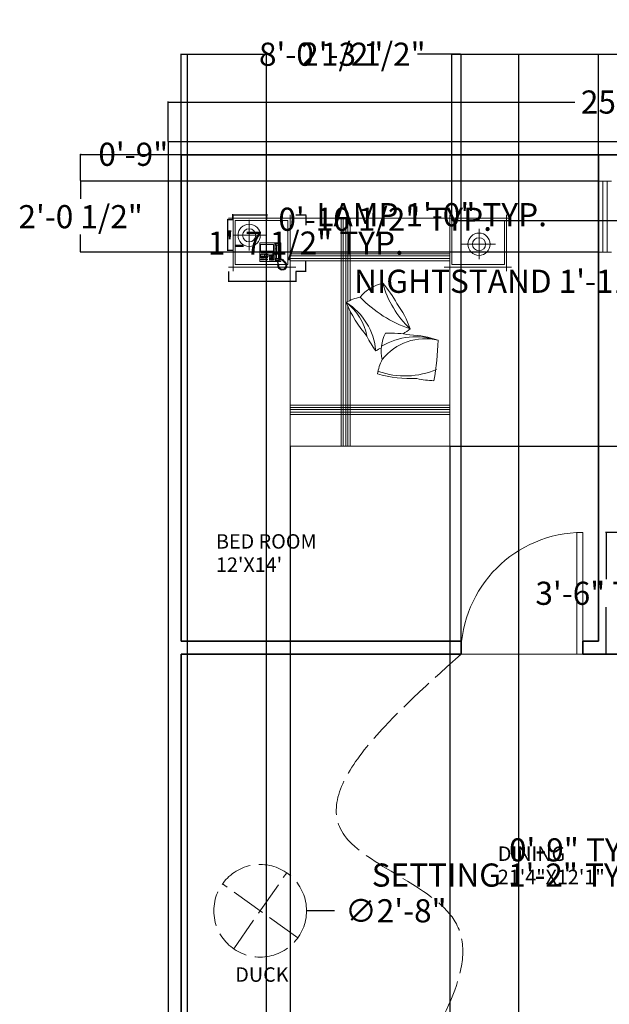
# Model space of a CAD drawing. Units: inches. Extents: x -26 to 385, y 12 to 697.
# Tile 12 of 13: x -26 to 177, y 356 to 697. Entities that reach past the tile are written whole.
import ezdxf

# ---------------------------------------------------------------- set-up
doc = ezdxf.new("R2010")
doc.units = ezdxf.units.IN
doc.header["$MEASUREMENT"] = 0
doc.linetypes.add('ACAD_ISO02W100', pattern=[15, 12, -3])
for name, color, linetype, lineweight in [('A-ANNO-DIMS', 4, 'Continuous', 18), ('A-AREA-IDEN', 4, 'Continuous', 18), ('A-DOOR', 30, 'Continuous', 20), ('A-EQPM', 210, 'Continuous', 13), ('A-FLOR-OVHD', 3, 'ACAD_ISO02W100', 13), ('A-GLAZ', 5, 'Continuous', 18), ('A-WALL', 40, 'Continuous', 35), ('C-PROP', 40, 'Continuous', 25), ('Furniture', 210, 'Continuous', 15)]:
    doc.layers.add(name, color=color, linetype=linetype, lineweight=lineweight)
doc.styles.get("Standard").update_dxf_attribs({"font": 'italic8.shx'})
doc.dimstyles.get("Standard").update_dxf_attribs({"dimtxt": 8, "dimasz": 0.18, "dimexe": 0.18, "dimexo": 0.0625, "dimgap": 0.09, "dimtad": 0, "dimtih": 1, "dimtoh": 1, "dimdec": 4, "dimzin": 0, "dimdsep": 46, "dimlunit": 3, "dimtxsty": 'Standard', "dimcen": 0.09, "dimclrd": 2, "dimclre": 3, "dimclrt": 6, "dimadec": 0, "dimazin": 0, "dimtfac": 1, "dimtdec": 4, "dimtofl": 0, "dimtmove": 0, "dimatfit": 3, "dimfxl": 1, "dimtolj": 1, "dimtzin": 0, "dimarcsym": 0})

# ---------------------------------------------------------------- blocks, each defined once
blk = doc.blocks.new('*D1')
at = {"layer": 'A-ANNO-DIMS', "color": 0, "lineweight": -2, "transparency": 16777216}
for p, q in [((25.13, 654.44), (25.13, 668.29)), ((25.31, 668.11), (165.52, 668.11)), ((324.95, 668.11), (184.74, 668.11)), ((325.13, 654.44), (325.13, 668.29))]:
    blk.add_line(p, q, dxfattribs=at)
at = {"layer": 'A-ANNO-DIMS', "color": 0, "transparency": 16777216}
for points in [[(25.31, 668.14), (25.31, 668.08), (25.13, 668.11)], [(324.95, 668.14), (324.95, 668.08), (325.13, 668.11)]]:
    blk.add_solid(points, dxfattribs=at)
at = {"layer": 'Defpoints', "color": 0, "transparency": 16777216}
for p in [(325.13, 668.11), (25.13, 654.38), (325.13, 654.38)]:
    blk.add_point(p, dxfattribs=at)
at = {"layer": 'A-ANNO-DIMS', "color": 0, "transparency": 16777216, "insert": (175.13, 668.11), "char_height": 8, "attachment_point": 5}
blk.add_mtext("\\A1;25'", dxfattribs=at)
blk = doc.blocks.new('DOOR-SWING-42IN')
for p, q in [((0, 0), (0, 42)), ((2, 0), (2, 42)), ((42, 0), (0, 0))]:
    blk.add_line(p, q)
blk.add_arc((0, 0), 42, 0, 90)
blk = doc.blocks.new('LAMP-BEDSIDE')
for p, q in [((0, -5.2), (0, 5.37)), ((-5.64, 0), (6.16, 0))]:
    blk.add_line(p, q)
for radius in [3.85, 2.27]:
    blk.add_circle((0, 0), radius)
blk = doc.blocks.new('NIGHTSTAND')
for p, q in [((-0.72, 17.12), (-0.72, -2.31)), ((18.22, 15.18), (0, 15.18)), ((0, 15.18), (0, 0)), ((18.22, 0), (18.22, 15.18)), ((0, 0), (18.22, 0)), ((-2.34, -0.93), (20.89, -0.93))]:
    blk.add_line(p, q)
blk = doc.blocks.new('*D15')
at = {"layer": 'A-ANNO-DIMS', "color": 3, "lineweight": -2, "transparency": 16777216}
for p, q in [((221.9, 409.73), (222.99, 407.84)), ((209.98, 402.84), (211.07, 400.96))]:
    blk.add_line(p, q, dxfattribs=at)
at = {"layer": 'A-ANNO-DIMS', "color": 2, "lineweight": -2, "transparency": 16777216}
for p, q in [((222.74, 407.9), (211.14, 401.2)), ((210.82, 401.02), (210.64, 401.02)), ((210.98, 401.11), (210.82, 401.02))]:
    blk.add_line(p, q, dxfattribs=at)
at = {"layer": 'A-ANNO-DIMS', "color": 2, "transparency": 16777216}
for points in [[(222.73, 407.93), (222.76, 407.88), (222.9, 407.99)], [(211.12, 401.23), (211.15, 401.18), (210.98, 401.11)]]:
    blk.add_solid(points, dxfattribs=at)
at = {"layer": 'Defpoints', "color": 0, "transparency": 16777216}
for p in [(221.87, 409.78), (209.95, 402.9), (210.98, 401.11)]:
    blk.add_point(p, dxfattribs=at)
at = {"layer": 'A-ANNO-DIMS', "color": 6, "transparency": 16777216, "insert": (143.32, 401.02), "char_height": 8, "attachment_point": 5}
blk.add_mtext('\\A1;SETTING 1\'-2" TYP.', dxfattribs=at)
blk = doc.blocks.new('*D16')
at = {"layer": 'A-ANNO-DIMS', "color": 2, "lineweight": -2, "transparency": 16777216}
for p, q in [((203.62, 409.73), (203.44, 409.73)), ((203.71, 409.58), (203.62, 409.73)), ((208.07, 402.02), (203.8, 409.42))]:
    blk.add_line(p, q, dxfattribs=at)
at = {"layer": 'A-ANNO-DIMS', "color": 3, "lineweight": -2, "transparency": 16777216}
for p, q in [((205.44, 410.58), (203.55, 409.49)), ((209.89, 402.87), (208, 401.78))]:
    blk.add_line(p, q, dxfattribs=at)
at = {"layer": 'A-ANNO-DIMS', "color": 2, "transparency": 16777216}
for points in [[(203.82, 409.44), (203.77, 409.41), (203.71, 409.58)], [(208.1, 402.04), (208.04, 402.01), (208.16, 401.87)]]:
    blk.add_solid(points, dxfattribs=at)
at = {"layer": 'Defpoints', "color": 0, "transparency": 16777216}
for p in [(203.71, 409.58), (205.5, 410.61), (209.95, 402.9)]:
    blk.add_point(p, dxfattribs=at)
at = {"layer": 'A-ANNO-DIMS', "color": 6, "transparency": 16777216, "insert": (167.16, 409.73), "char_height": 8, "attachment_point": 5}
blk.add_mtext('\\A1;0\'-9" TYP.', dxfattribs=at)
blk = doc.blocks.new('*D20')
at = {"layer": 'A-ANNO-DIMS', "color": 3, "lineweight": -2, "transparency": 16777216}
for p, q in [((182.53, 519.38), (176.11, 519.38)), ((182.53, 477.38), (176.11, 477.38))]:
    blk.add_line(p, q, dxfattribs=at)
at = {"layer": 'A-ANNO-DIMS', "color": 2, "lineweight": -2, "transparency": 16777216}
for p, q in [((176.29, 519.2), (176.29, 503.23)), ((176.29, 477.56), (176.29, 493.53))]:
    blk.add_line(p, q, dxfattribs=at)
at = {"layer": 'A-ANNO-DIMS', "color": 2, "transparency": 16777216}
for points in [[(176.26, 519.2), (176.32, 519.2), (176.29, 519.38)], [(176.26, 477.56), (176.32, 477.56), (176.29, 477.38)]]:
    blk.add_solid(points, dxfattribs=at)
at = {"layer": 'Defpoints', "color": 0, "transparency": 16777216}
for p in [(176.29, 519.38), (182.59, 519.38), (182.59, 477.38)]:
    blk.add_point(p, dxfattribs=at)
at = {"layer": 'A-ANNO-DIMS', "color": 6, "transparency": 16777216, "insert": (176.29, 498.38), "char_height": 8, "attachment_point": 5}
blk.add_mtext('\\A1;3\'-6" TYP.', dxfattribs=at)
blk = doc.blocks.new('*D21')
at = {"layer": 'A-ANNO-DIMS', "color": 3, "lineweight": -2, "transparency": 16777216}
for p, q in [((45.89, 609.6), (45.89, 606)), ((69.11, 609.6), (69.11, 606))]:
    blk.add_line(p, q, dxfattribs=at)
at = {"layer": 'A-ANNO-DIMS', "color": 2, "lineweight": -2, "transparency": 16777216}
for p, q in [((46.07, 606.18), (68.93, 606.18)), ((69.11, 606.18), (69.29, 606.18))]:
    blk.add_line(p, q, dxfattribs=at)
at = {"layer": 'A-ANNO-DIMS', "color": 2, "transparency": 16777216}
for points in [[(46.07, 606.21), (46.07, 606.15), (45.89, 606.18)], [(68.93, 606.21), (68.93, 606.15), (69.11, 606.18)]]:
    blk.add_solid(points, dxfattribs=at)
at = {"layer": 'Defpoints', "color": 0, "transparency": 16777216}
for p in [(45.89, 609.66), (69.11, 609.66), (69.11, 606.18)]:
    blk.add_point(p, dxfattribs=at)
at = {"layer": 'A-ANNO-DIMS', "color": 6, "transparency": 16777216, "insert": (152.05, 606.18), "char_height": 8, "attachment_point": 5}
blk.add_mtext('\\A1;NIGHTSTAND 1\'-11" TYP.', dxfattribs=at)
blk = doc.blocks.new('*D22')
at = {"layer": 'A-ANNO-DIMS', "color": 3, "lineweight": -2, "transparency": 16777216}
for p, q in [((69.18, 629.09), (72.78, 629.09)), ((69.18, 609.66), (72.78, 609.66))]:
    blk.add_line(p, q, dxfattribs=at)
at = {"layer": 'A-ANNO-DIMS', "color": 2, "lineweight": -2, "transparency": 16777216}
for p, q in [((72.6, 628.91), (72.6, 625.56)), ((72.6, 609.84), (72.6, 613.19))]:
    blk.add_line(p, q, dxfattribs=at)
at = {"layer": 'A-ANNO-DIMS', "color": 2, "transparency": 16777216}
for points in [[(72.57, 628.91), (72.63, 628.91), (72.6, 629.09)], [(72.57, 609.84), (72.63, 609.84), (72.6, 609.66)]]:
    blk.add_solid(points, dxfattribs=at)
at = {"layer": 'Defpoints', "color": 0, "transparency": 16777216}
for p in [(69.11, 629.09), (72.6, 629.09), (69.11, 609.66)]:
    blk.add_point(p, dxfattribs=at)
at = {"layer": 'A-ANNO-DIMS', "color": 6, "transparency": 16777216, "insert": (72.6, 619.37), "char_height": 8, "attachment_point": 5}
blk.add_mtext('\\A1;1\'-7 1/2" TYP.', dxfattribs=at)
blk = doc.blocks.new('*D23')
at = {"layer": 'A-ANNO-DIMS', "color": 3, "lineweight": -2, "transparency": 16777216}
for p, q in [((47.41, 627.49), (47.41, 629.37)), ((59.21, 627.49), (59.21, 629.37))]:
    blk.add_line(p, q, dxfattribs=at)
at = {"layer": 'A-ANNO-DIMS', "color": 2, "lineweight": -2, "transparency": 16777216}
for p, q in [((47.59, 629.19), (59.03, 629.19)), ((59.21, 629.19), (59.39, 629.19))]:
    blk.add_line(p, q, dxfattribs=at)
at = {"layer": 'A-ANNO-DIMS', "color": 2, "transparency": 16777216}
for points in [[(47.59, 629.22), (47.59, 629.16), (47.41, 629.19)], [(59.03, 629.22), (59.03, 629.16), (59.21, 629.19)]]:
    blk.add_solid(points, dxfattribs=at)
at = {"layer": 'Defpoints', "color": 0, "transparency": 16777216}
for p in [(47.41, 627.43), (59.21, 629.19), (59.21, 627.43)]:
    blk.add_point(p, dxfattribs=at)
at = {"layer": 'A-ANNO-DIMS', "color": 6, "transparency": 16777216, "insert": (116.05, 629.19), "char_height": 8, "attachment_point": 5}
blk.add_mtext('\\A1;LAMP 1\'-0" TYP.', dxfattribs=at)
blk = doc.blocks.new('*D24')
at = {"layer": 'A-ANNO-DIMS', "color": 3, "lineweight": -2, "transparency": 16777216}
for p, q in [((47.35, 627.43), (45.46, 627.43)), ((47.35, 616.86), (45.46, 616.86))]:
    blk.add_line(p, q, dxfattribs=at)
at = {"layer": 'A-ANNO-DIMS', "color": 2, "lineweight": -2, "transparency": 16777216}
for p, q in [((45.64, 627.43), (45.64, 627.61)), ((45.64, 627.61), (45.82, 627.61)), ((45.64, 617.04), (45.64, 627.25))]:
    blk.add_line(p, q, dxfattribs=at)
at = {"layer": 'A-ANNO-DIMS', "color": 2, "transparency": 16777216}
for points in [[(45.61, 627.25), (45.67, 627.25), (45.64, 627.43)], [(45.61, 617.04), (45.67, 617.04), (45.64, 616.86)]]:
    blk.add_solid(points, dxfattribs=at)
at = {"layer": 'Defpoints', "color": 0, "transparency": 16777216}
for p in [(45.64, 627.43), (47.41, 627.43), (47.41, 616.86)]:
    blk.add_point(p, dxfattribs=at)
at = {"layer": 'A-ANNO-DIMS', "color": 6, "transparency": 16777216, "insert": (100.01, 627.61), "char_height": 8, "attachment_point": 5}
blk.add_mtext('\\A1;0\'-10 1/2" TYP.', dxfattribs=at)
blk = doc.blocks.new('*D29')
at = {"layer": 'A-ANNO-DIMS', "color": 3, "lineweight": -2, "transparency": 16777216}
for p, q in [((67.17, 549.17), (67.17, 23.95)), ((122.29, 549.17), (122.29, 23.95))]:
    blk.add_line(p, q, dxfattribs=at)
at = {"layer": 'A-ANNO-DIMS', "color": 2, "lineweight": -2, "transparency": 16777216}
for p, q in [((67.35, 24.13), (76.92, 24.13)), ((122.11, 24.13), (112.53, 24.13))]:
    blk.add_line(p, q, dxfattribs=at)
at = {"layer": 'A-ANNO-DIMS', "color": 2, "transparency": 16777216}
for points in [[(67.35, 24.16), (67.35, 24.1), (67.17, 24.13)], [(122.11, 24.16), (122.11, 24.1), (122.29, 24.13)]]:
    blk.add_solid(points, dxfattribs=at)
at = {"layer": 'Defpoints', "color": 0, "transparency": 16777216}
for p in [(67.17, 549.23), (122.29, 549.23), (122.29, 24.13)]:
    blk.add_point(p, dxfattribs=at)
at = {"layer": 'A-ANNO-DIMS', "color": 6, "transparency": 16777216, "insert": (94.73, 24.13), "char_height": 8, "attachment_point": 5}
blk.add_mtext('\\A1;4\'-7"', dxfattribs=at)
blk = doc.blocks.new('*D30')
at = {"layer": 'A-ANNO-DIMS', "color": 3, "lineweight": -2, "transparency": 16777216}
for p, q in [((123.07, 627.15), (355.56, 627.15)), ((122.35, 549.23), (355.56, 549.23))]:
    blk.add_line(p, q, dxfattribs=at)
at = {"layer": 'A-ANNO-DIMS', "color": 2, "lineweight": -2, "transparency": 16777216}
for p, q in [((355.38, 626.97), (355.38, 593.04)), ((355.38, 549.41), (355.38, 583.34))]:
    blk.add_line(p, q, dxfattribs=at)
at = {"layer": 'A-ANNO-DIMS', "color": 2, "transparency": 16777216}
for points in [[(355.35, 626.97), (355.41, 626.97), (355.38, 627.15)], [(355.35, 549.41), (355.41, 549.41), (355.38, 549.23)]]:
    blk.add_solid(points, dxfattribs=at)
at = {"layer": 'Defpoints', "color": 0, "transparency": 16777216}
for p in [(123.01, 627.15), (122.29, 549.23), (355.38, 549.23)]:
    blk.add_point(p, dxfattribs=at)
at = {"layer": 'A-ANNO-DIMS', "color": 6, "transparency": 16777216, "insert": (355.38, 588.19), "char_height": 8, "attachment_point": 5}
blk.add_mtext('\\A1;6\'-6"', dxfattribs=at)
blk = doc.blocks.new('*D36')
at = {"layer": 'A-ANNO-DIMS', "color": 3, "lineweight": -2, "transparency": 16777216}
for p, q in [((146.13, 147.94), (146.13, 684.81)), ((193.6, 147.94), (193.6, 684.81))]:
    blk.add_line(p, q, dxfattribs=at)
at = {"layer": 'A-ANNO-DIMS', "color": 2, "lineweight": -2, "transparency": 16777216}
for p, q in [((146.31, 684.63), (193.42, 684.63)), ((193.6, 684.63), (193.78, 684.63))]:
    blk.add_line(p, q, dxfattribs=at)
at = {"layer": 'A-ANNO-DIMS', "color": 2, "transparency": 16777216}
for points in [[(146.31, 684.66), (146.31, 684.6), (146.13, 684.63)], [(193.42, 684.66), (193.42, 684.6), (193.6, 684.63)]]:
    blk.add_solid(points, dxfattribs=at)
at = {"layer": 'Defpoints', "color": 0, "transparency": 16777216}
for p in [(193.6, 684.63), (146.13, 147.88), (193.6, 147.88)]:
    blk.add_point(p, dxfattribs=at)
at = {"layer": 'A-ANNO-DIMS', "color": 6, "transparency": 16777216, "insert": (228.34, 684.63), "char_height": 8, "attachment_point": 5}
blk.add_mtext('\\A1;3\'-11 1/2"', dxfattribs=at)
blk = doc.blocks.new('*D38')
at = {"layer": 'A-ANNO-DIMS', "color": 3, "lineweight": -2, "transparency": 16777216}
for p, q in [((173.57, 640.78), (-5.3, 640.78)), ((173.57, 616.23), (-5.3, 616.23))]:
    blk.add_line(p, q, dxfattribs=at)
at = {"layer": 'A-ANNO-DIMS', "color": 2, "lineweight": -2, "transparency": 16777216}
for p, q in [((-5.12, 640.6), (-5.12, 634.69)), ((-5.12, 616.41), (-5.12, 622.32))]:
    blk.add_line(p, q, dxfattribs=at)
at = {"layer": 'A-ANNO-DIMS', "color": 2, "transparency": 16777216}
for points in [[(-5.15, 640.6), (-5.09, 640.6), (-5.12, 640.78)], [(-5.15, 616.41), (-5.09, 616.41), (-5.12, 616.23)]]:
    blk.add_solid(points, dxfattribs=at)
at = {"layer": 'Defpoints', "color": 0, "transparency": 16777216}
for p in [(-5.12, 640.78), (173.63, 640.78), (173.63, 616.23)]:
    blk.add_point(p, dxfattribs=at)
at = {"layer": 'A-ANNO-DIMS', "color": 6, "transparency": 16777216, "insert": (-5.12, 628.5), "char_height": 8, "attachment_point": 5}
blk.add_mtext('\\A1;2\'-0 1/2"', dxfattribs=at)
blk = doc.blocks.new('*D41')
at = {"layer": 'A-ANNO-DIMS', "color": 3, "lineweight": -2, "transparency": 16777216}
for p, q in [((31.81, 313.9), (31.81, 684.81)), ((59.08, 304.23), (59.08, 684.81))]:
    blk.add_line(p, q, dxfattribs=at)
at = {"layer": 'A-ANNO-DIMS', "color": 2, "lineweight": -2, "transparency": 16777216}
for p, q in [((31.99, 684.63), (58.9, 684.63)), ((59.08, 684.63), (59.26, 684.63))]:
    blk.add_line(p, q, dxfattribs=at)
at = {"layer": 'A-ANNO-DIMS', "color": 2, "transparency": 16777216}
for points in [[(31.99, 684.66), (31.99, 684.6), (31.81, 684.63)], [(58.9, 684.66), (58.9, 684.6), (59.08, 684.63)]]:
    blk.add_solid(points, dxfattribs=at)
at = {"layer": 'Defpoints', "color": 0, "transparency": 16777216}
for p in [(59.08, 684.63), (31.81, 313.84), (59.08, 304.16)]:
    blk.add_point(p, dxfattribs=at)
at = {"layer": 'A-ANNO-DIMS', "color": 6, "transparency": 16777216, "insert": (92.49, 684.63), "char_height": 8, "attachment_point": 5}
blk.add_mtext('\\A1;2\'-3 1/2"', dxfattribs=at)
blk = doc.blocks.new('*D45')
at = {"layer": 'A-ANNO-DIMS', "color": 3, "lineweight": -2, "transparency": 16777216}
for p, q in [((29.63, 481.94), (29.63, 684.81)), ((126.2, 481.94), (126.2, 684.81))]:
    blk.add_line(p, q, dxfattribs=at)
at = {"layer": 'A-ANNO-DIMS', "color": 2, "lineweight": -2, "transparency": 16777216}
for p, q in [((29.81, 684.63), (44.68, 684.63)), ((126.02, 684.63), (111.15, 684.63))]:
    blk.add_line(p, q, dxfattribs=at)
at = {"layer": 'A-ANNO-DIMS', "color": 2, "transparency": 16777216}
for points in [[(29.81, 684.66), (29.81, 684.6), (29.63, 684.63)], [(126.02, 684.66), (126.02, 684.6), (126.2, 684.63)]]:
    blk.add_solid(points, dxfattribs=at)
at = {"layer": 'Defpoints', "color": 0, "transparency": 16777216}
for p in [(126.2, 684.63), (29.63, 481.88), (126.2, 481.88)]:
    blk.add_point(p, dxfattribs=at)
at = {"layer": 'A-ANNO-DIMS', "color": 6, "transparency": 16777216, "insert": (77.91, 684.63), "char_height": 8, "attachment_point": 5}
blk.add_mtext('\\A1;8\'-0 1/2"', dxfattribs=at)
blk = doc.blocks.new('*D48')
at = {"layer": 'A-ANNO-DIMS', "color": 3, "lineweight": -2, "transparency": 16777216}
for p, q in [((123.01, 627.21), (123.01, 684.81)), ((173.63, 649.94), (173.63, 684.81))]:
    blk.add_line(p, q, dxfattribs=at)
at = {"layer": 'A-ANNO-DIMS', "color": 2, "lineweight": -2, "transparency": 16777216}
for p, q in [((123.19, 684.63), (173.45, 684.63)), ((173.63, 684.63), (173.81, 684.63))]:
    blk.add_line(p, q, dxfattribs=at)
at = {"layer": 'A-ANNO-DIMS', "color": 2, "transparency": 16777216}
for points in [[(123.19, 684.66), (123.19, 684.6), (123.01, 684.63)], [(173.45, 684.66), (173.45, 684.6), (173.63, 684.63)]]:
    blk.add_solid(points, dxfattribs=at)
at = {"layer": 'Defpoints', "color": 0, "transparency": 16777216}
for p in [(173.63, 684.63), (173.63, 649.88), (123.01, 627.15)]:
    blk.add_point(p, dxfattribs=at)
at = {"layer": 'A-ANNO-DIMS', "color": 6, "transparency": 16777216, "insert": (207.04, 684.63), "char_height": 8, "attachment_point": 5}
blk.add_mtext('\\A1;4\'-2 1/2"', dxfattribs=at)
blk = doc.blocks.new('*D49')
at = {"layer": 'A-ANNO-DIMS', "color": 3, "lineweight": -2, "transparency": 16777216}
for p, q in [((173.69, 649.88), (355.56, 649.88)), ((123.07, 627.15), (355.56, 627.15))]:
    blk.add_line(p, q, dxfattribs=at)
at = {"layer": 'A-ANNO-DIMS', "color": 2, "lineweight": -2, "transparency": 16777216}
for p, q in [((355.38, 649.7), (355.38, 644.7)), ((355.38, 627.33), (355.38, 632.33))]:
    blk.add_line(p, q, dxfattribs=at)
at = {"layer": 'A-ANNO-DIMS', "color": 2, "transparency": 16777216}
for points in [[(355.35, 649.7), (355.41, 649.7), (355.38, 649.88)], [(355.35, 627.33), (355.41, 627.33), (355.38, 627.15)]]:
    blk.add_solid(points, dxfattribs=at)
at = {"layer": 'Defpoints', "color": 0, "transparency": 16777216}
for p in [(173.63, 649.88), (355.38, 649.88), (123.01, 627.15)]:
    blk.add_point(p, dxfattribs=at)
at = {"layer": 'A-ANNO-DIMS', "color": 6, "transparency": 16777216, "insert": (355.38, 638.52), "char_height": 8, "attachment_point": 5}
blk.add_mtext('\\A1;1\'-10 1/2"', dxfattribs=at)
blk = doc.blocks.new('*D54')
at = {"layer": 'A-ANNO-DIMS', "color": 3, "lineweight": -2, "transparency": 16777216}
for p, q in [((173.57, 649.88), (-5.3, 649.88)), ((173.57, 640.78), (-5.3, 640.78))]:
    blk.add_line(p, q, dxfattribs=at)
at = {"layer": 'A-ANNO-DIMS', "color": 2, "lineweight": -2, "transparency": 16777216}
for p, q in [((-5.12, 649.88), (-5.12, 650.06)), ((-5.12, 650.06), (-4.94, 650.06)), ((-5.12, 640.96), (-5.12, 649.7))]:
    blk.add_line(p, q, dxfattribs=at)
at = {"layer": 'A-ANNO-DIMS', "color": 2, "transparency": 16777216}
for points in [[(-5.15, 649.7), (-5.09, 649.7), (-5.12, 649.88)], [(-5.15, 640.96), (-5.09, 640.96), (-5.12, 640.78)]]:
    blk.add_solid(points, dxfattribs=at)
at = {"layer": 'Defpoints', "color": 0, "transparency": 16777216}
for p in [(-5.12, 649.88), (173.63, 649.88), (173.63, 640.78)]:
    blk.add_point(p, dxfattribs=at)
at = {"layer": 'A-ANNO-DIMS', "color": 6, "transparency": 16777216, "insert": (13.05, 650.06), "char_height": 8, "attachment_point": 5}
blk.add_mtext('\\A1;0\'-9"', dxfattribs=at)
blk = doc.blocks.new('*D57')
at = {"layer": 'A-ANNO-DIMS', "color": 3, "lineweight": -2, "transparency": 16777216}
for p, q in [((56.77, 388.68), (56.95, 388.68)), ((56.86, 388.59), (56.86, 388.77))]:
    blk.add_line(p, q, dxfattribs=at)
at = {"layer": 'A-ANNO-DIMS', "color": 2, "lineweight": -2, "transparency": 16777216}
blk.add_line((82.47, 388.68), (73.05, 388.68), dxfattribs=at)
at = {"layer": 'A-ANNO-DIMS', "color": 2, "transparency": 16777216}
blk.add_solid([(73.05, 388.71), (73.05, 388.65), (72.87, 388.68)], dxfattribs=at)
at = {"layer": 'Defpoints', "color": 0, "transparency": 16777216}
for p in [(40.85, 388.68), (72.87, 388.68)]:
    blk.add_point(p, dxfattribs=at)
at = {"layer": 'A-ANNO-DIMS', "color": 6, "transparency": 16777216, "insert": (103.7, 388.68), "char_height": 8, "attachment_point": 5}
blk.add_mtext('\\A1;∅2\'-8"', dxfattribs=at)

msp = doc.modelspace()

# ---------------------------------------------------------------- linework, layer by layer
at = {"layer": 'A-EQPM'}
for p, q in [((56.83045, 619.43254), (56.74045, 619.34254)), ((56.74045, 619.34254), (56.74045, 613.13255)), ((56.83045, 619.43254), (63.94044, 619.43254)), ((61.91544, 619.07254), (62.09544, 619.29754)), ((62.09544, 619.16254), (62.05044, 618.98254)), ((62.09544, 619.29754), (63.44544, 619.29754)), ((62.27544, 619.25254), (62.09544, 619.16254)), ((62.27544, 619.25254), (63.35544, 619.25254)), ((62.50044, 618.66754), (62.27544, 619.25254)), ((63.13044, 618.66754), (63.35544, 619.25254)), ((63.35544, 619.25254), (63.53544, 619.16254)), ((63.44544, 619.29754), (63.67044, 619.07254)), ((63.53544, 619.16254), (63.58044, 618.98254)), ((63.94044, 619.43254), (64.03043, 619.34254)), ((64.03043, 619.34254), (64.03043, 613.13255)), ((61.51044, 618.93754), (57.01045, 618.93754)), ((57.01045, 618.93754), (57.01045, 616.55254)), ((57.01045, 616.55254), (61.51044, 616.55254)), ((61.51044, 616.46254), (57.19045, 616.46254)), ((57.19045, 616.46254), (57.19045, 616.01254)), ((57.19045, 616.18147), (61.51044, 616.18147)), ((57.19045, 616.01254), (61.51044, 616.01254)), ((57.55045, 616.46254), (57.55045, 616.01254)), ((57.91045, 616.46254), (57.91045, 616.01254)), ((58.27045, 616.46254), (58.27045, 616.01254)), ((58.63045, 616.46254), (58.63045, 616.01254)), ((58.99045, 616.46254), (58.99045, 616.01254)), ((59.31975, 616.01254), (59.48871, 616.1815)), ((59.35044, 616.46254), (59.35044, 616.01254)), ((61.51044, 616.55254), (61.51044, 618.93754)), ((61.51044, 616.01254), (61.51044, 616.46254)), ((61.91544, 613.62755), (61.91544, 619.07254)), ((61.91544, 616.18147), (62.32044, 616.18147)), ((62.05044, 618.98254), (62.05044, 617.76754)), ((62.05044, 618.98254), (62.45544, 618.57754)), ((62.05044, 617.76754), (62.14044, 617.54254)), ((62.14044, 617.54254), (62.27544, 617.31754)), ((62.27544, 617.31754), (62.32044, 617.00254)), ((62.32044, 615.69754), (62.32044, 617.00254)), ((62.45544, 618.57754), (62.50044, 618.66754)), ((62.45544, 618.57754), (62.45544, 614.12255)), ((63.13044, 618.66754), (62.50044, 618.66754)), ((63.17544, 618.57754), (63.13044, 618.66754)), ((63.58044, 618.98254), (63.17544, 618.57754)), ((63.17544, 618.57754), (63.17544, 614.12255)), ((63.35544, 617.31754), (63.31044, 617.00254)), ((63.31044, 615.69754), (63.31044, 617.00254)), ((63.49044, 617.54254), (63.35544, 617.31754)), ((63.58044, 617.76754), (63.49044, 617.54254)), ((63.58044, 618.98254), (63.58044, 617.76754)), ((63.67044, 619.07254), (63.67044, 613.67255)), ((56.74045, 613.13255), (56.83045, 613.04255)), ((62.81317, 613.04255), (56.83045, 613.04255)), ((59.66544, 615.51754), (57.01045, 615.51754)), ((57.01045, 615.51754), (57.01045, 614.70754)), ((57.01045, 614.70754), (59.66544, 614.70754)), ((57.05545, 614.48255), (57.05545, 614.30255)), ((57.50545, 614.48255), (57.05545, 614.48255)), ((57.05545, 614.30255), (57.50545, 614.30255)), ((57.05545, 613.80755), (57.50545, 613.80755)), ((57.05545, 613.53755), (57.05545, 613.80755)), ((57.05545, 613.74824), (57.11476, 613.80755)), ((57.50545, 613.53755), (57.05545, 613.53755)), ((57.46045, 615.42754), (57.46045, 615.29254)), ((57.59545, 615.42754), (57.46045, 615.42754)), ((57.46045, 615.29254), (57.59545, 615.29254)), ((57.46045, 614.93254), (57.46045, 614.79754)), ((57.59545, 614.93254), (57.46045, 614.93254)), ((57.46045, 614.79754), (57.59545, 614.79754)), ((57.50545, 614.30255), (57.50545, 614.48255)), ((57.50545, 613.80755), (57.50545, 613.53755)), ((57.59545, 615.29254), (57.59545, 615.42754)), ((57.59545, 614.79754), (57.59545, 614.93254)), ((57.68545, 614.48255), (57.68545, 614.30255)), ((58.13545, 614.48255), (57.68545, 614.48255)), ((57.68545, 614.37824), (57.78976, 614.48255)), ((57.68545, 614.30255), (58.13545, 614.30255)), ((57.68545, 613.80755), (58.13545, 613.80755)), ((57.68545, 613.53755), (57.68545, 613.80755)), ((58.13545, 613.53755), (57.68545, 613.53755)), ((58.01476, 614.70754), (58.82475, 615.51754)), ((58.13545, 614.30255), (58.13545, 614.48255)), ((58.13545, 613.80755), (58.13545, 613.53755)), ((58.40545, 615.42754), (58.27045, 615.42754)), ((58.27045, 615.42754), (58.27045, 615.29254)), ((58.27045, 615.29254), (58.40545, 615.29254)), ((58.40545, 614.93254), (58.27045, 614.93254)), ((58.27045, 614.93254), (58.27045, 614.79754)), ((58.27045, 614.79754), (58.40545, 614.79754)), ((58.31545, 614.48255), (58.31545, 614.30255)), ((58.76545, 614.48255), (58.31545, 614.48255)), ((58.31545, 614.30255), (58.76545, 614.30255)), ((58.31545, 613.80755), (58.76545, 613.80755)), ((58.31545, 613.53755), (58.31545, 613.80755)), ((58.76545, 613.53755), (58.31545, 613.53755)), ((58.40545, 615.29254), (58.40545, 615.42754)), ((58.40545, 614.79754), (58.40545, 614.93254)), ((58.76545, 614.30255), (58.76545, 614.48255)), ((58.76545, 613.80755), (58.76545, 613.53755)), ((59.39544, 614.48255), (58.94545, 614.48255)), ((58.94545, 614.48255), (58.94545, 614.30255)), ((58.94545, 614.30255), (59.39544, 614.30255)), ((58.94545, 613.53755), (58.94545, 613.80755)), ((58.94545, 613.80755), (59.39544, 613.80755)), ((59.39544, 613.53755), (58.94545, 613.53755)), ((59.21544, 615.42754), (59.08044, 615.42754)), ((59.08044, 615.42754), (59.08044, 615.29254)), ((59.08044, 615.29254), (59.21544, 615.29254)), ((59.21544, 614.93254), (59.08044, 614.93254)), ((59.08044, 614.93254), (59.08044, 614.79754)), ((59.08044, 614.79754), (59.21544, 614.79754)), ((59.21544, 615.29254), (59.21544, 615.42754)), ((59.21544, 614.79754), (59.21544, 614.93254)), ((59.39544, 614.30255), (59.39544, 614.48255)), ((59.39544, 613.80755), (59.39544, 613.53755)), ((59.66544, 614.70754), (59.66544, 615.51754)), ((60.07044, 615.02254), (60.07044, 615.29254)), ((60.07044, 615.29254), (60.43044, 615.29254)), ((60.43044, 615.02254), (60.07044, 615.02254)), ((60.07044, 614.52755), (60.07044, 614.79754)), ((60.07044, 614.79754), (60.43044, 614.79754)), ((60.43044, 614.52755), (60.07044, 614.52755)), ((60.07044, 613.98755), (60.07044, 614.25755)), ((60.07044, 614.25755), (60.43044, 614.25755)), ((60.43044, 613.98755), (60.07044, 613.98755)), ((60.07044, 613.49255), (60.07044, 613.76255)), ((60.07044, 613.76255), (60.43044, 613.76255)), ((60.43044, 613.49255), (60.07044, 613.49255)), ((60.43044, 615.29254), (60.43044, 615.02254)), ((60.43044, 614.79754), (60.43044, 614.52755)), ((60.43044, 614.25755), (60.43044, 613.98755)), ((60.43044, 613.76255), (60.43044, 613.49255)), ((60.61044, 615.29254), (60.97044, 615.29254)), ((60.61044, 615.02254), (60.61044, 615.29254)), ((60.97044, 615.02254), (60.61044, 615.02254)), ((60.61044, 614.52755), (60.61044, 614.79754)), ((60.61044, 614.79754), (60.97044, 614.79754)), ((60.97044, 614.52755), (60.61044, 614.52755)), ((60.61044, 614.25755), (60.97044, 614.25755)), ((60.61044, 613.98755), (60.61044, 614.25755)), ((60.97044, 613.98755), (60.61044, 613.98755)), ((60.61044, 613.49255), (60.61044, 613.76255)), ((60.61044, 613.76255), (60.97044, 613.76255)), ((60.97044, 613.49255), (60.61044, 613.49255)), ((60.97044, 615.29254), (60.97044, 615.02254)), ((60.97044, 614.79754), (60.97044, 614.52755)), ((60.97044, 614.25755), (60.97044, 613.98755)), ((60.97044, 613.76255), (60.97044, 613.49255)), ((61.15044, 615.02254), (61.15044, 615.29254)), ((61.15044, 615.29254), (61.51044, 615.29254)), ((61.51044, 615.02254), (61.15044, 615.02254)), ((61.15044, 614.52755), (61.15044, 614.79754)), ((61.15044, 614.79754), (61.51044, 614.79754)), ((61.51044, 614.52755), (61.15044, 614.52755)), ((61.15044, 614.30255), (61.51044, 614.30255)), ((61.15044, 614.03255), (61.15044, 614.30255)), ((61.51044, 614.03255), (61.15044, 614.03255)), ((61.15044, 613.76255), (61.51044, 613.76255)), ((61.15044, 613.49255), (61.15044, 613.76255)), ((61.51044, 613.49255), (61.15044, 613.49255)), ((61.51044, 615.29254), (61.51044, 615.02254)), ((61.51044, 614.79754), (61.51044, 614.52755)), ((61.51044, 614.30255), (61.51044, 614.03255)), ((61.51044, 613.76255), (61.51044, 613.49255)), ((62.14044, 613.40255), (61.91544, 613.62755)), ((62.05044, 614.93254), (62.14044, 615.15754)), ((62.05044, 613.71755), (62.05044, 614.93254)), ((62.05044, 613.71755), (62.45544, 614.12255)), ((62.09544, 613.53755), (62.05044, 613.71755)), ((62.27544, 613.44755), (62.09544, 613.53755)), ((62.14044, 615.15754), (62.27544, 615.38254)), ((62.77336, 613.40255), (62.14044, 613.40255)), ((62.27544, 615.38254), (62.32044, 615.69754)), ((62.50044, 614.03255), (62.27544, 613.44755)), ((62.27544, 613.44755), (62.77263, 613.44755)), ((62.45544, 614.12255), (62.50044, 614.03255)), ((63.13044, 614.03255), (62.50044, 614.03255)), ((62.90544, 613.58255), (62.77044, 613.58255)), ((62.77044, 613.58255), (62.77673, 613.19448)), ((62.77673, 613.19448), (62.88601, 612.73886)), ((62.88601, 612.73886), (62.99529, 612.31057)), ((62.93154, 613.22182), (62.90544, 613.58255)), ((62.91521, 613.44755), (63.35544, 613.44755)), ((63.44544, 613.40255), (62.91846, 613.40255)), ((62.99529, 612.93022), (62.93154, 613.22182)), ((63.94044, 613.04255), (62.97074, 613.04255)), ((63.10457, 612.50193), (62.99529, 612.93022)), ((63.13189, 612.28323), (63.10457, 612.50193)), ((63.17544, 614.12255), (63.13044, 614.03255)), ((63.13044, 614.03255), (63.35544, 613.44755)), ((63.58044, 613.71755), (63.17544, 614.12255)), ((63.35544, 615.38254), (63.31044, 615.69754)), ((63.49044, 615.15754), (63.35544, 615.38254)), ((63.35544, 613.44755), (63.53544, 613.53755)), ((63.67044, 613.67255), (63.44544, 613.40255)), ((63.58044, 614.93254), (63.49044, 615.15754)), ((63.53544, 613.53755), (63.58044, 613.71755)), ((63.58044, 613.71755), (63.58044, 614.93254)), ((64.03043, 613.13255), (63.94044, 613.04255)), ((64.30052, 613.84211), (64.03043, 613.94255)), ((64.03043, 613.76255), (64.22918, 613.70728)), ((64.22918, 613.70728), (64.41148, 613.56452)), ((64.42734, 613.71521), (64.30052, 613.84211)), ((64.41148, 613.56452), (64.45904, 613.50107)), ((64.52245, 613.62797), (64.42734, 613.71521)), ((64.45904, 613.50107), (64.55416, 613.509)), ((64.55416, 613.509), (64.45904, 613.41383)), ((64.45904, 613.41383), (64.82365, 613.08864)), ((64.6889, 613.69142), (64.52245, 613.62797)), ((64.76817, 613.61211), (64.6889, 613.69142)), ((64.70476, 613.47728), (64.76817, 613.61211)), ((64.81573, 613.56452), (64.70476, 613.47728)), ((64.93462, 613.43762), (64.81573, 613.56452)), ((64.82365, 613.08864), (65.41812, 612.58105)), ((64.8395, 613.17589), (64.93462, 613.43762)), ((65.08522, 613.30279), (64.8395, 613.17589)), ((65.2913, 613.10451), (65.08522, 613.30279)), ((65.24374, 612.81898), (65.2913, 613.10451)), ((65.44983, 612.94588), (65.24374, 612.81898)), ((65.42681, 612.56572), (65.72733, 611.70914)), ((65.62421, 612.76346), (65.44983, 612.94588)), ((65.55287, 612.56518), (65.62421, 612.76346)), ((65.82751, 612.59306), (65.5543, 612.56572)), ((65.90947, 612.31968), (65.82751, 612.59306)), ((62.91333, 611.91873), (62.89512, 611.70003)), ((62.89512, 611.70003), (63.15921, 611.65447)), ((63.15921, 611.65447), (62.90422, 611.49956)), ((62.90422, 611.49956), (62.92244, 611.25352)), ((63.01351, 612.01897), (62.91333, 611.91873)), ((62.92244, 611.25352), (63.21386, 611.22618)), ((63.21386, 611.22618), (62.95887, 611.02571)), ((62.95887, 611.02571), (63.07725, 610.81612)), ((62.99529, 612.31057), (62.98619, 612.07364)), ((62.98619, 612.07364), (63.01351, 612.01897)), ((63.07725, 610.81612), (63.35046, 610.8708)), ((63.12279, 612.04631), (63.13189, 612.28323)), ((63.28671, 611.92784), (63.12279, 612.04631)), ((63.35046, 610.8708), (63.22296, 610.61565)), ((63.22296, 610.61565), (63.35956, 610.45162)), ((63.25028, 611.71826), (63.28671, 611.92784)), ((63.29582, 611.14417), (63.25028, 611.71826)), ((63.64188, 610.70677), (63.29582, 611.14417)), ((63.35956, 610.45162), (63.56902, 610.60653)), ((63.56902, 610.60653), (63.53259, 610.3605)), ((63.53259, 610.3605), (63.70562, 610.25115)), ((64.12454, 610.45162), (63.64188, 610.70677)), ((63.70562, 610.25115), (63.92419, 610.4334)), ((63.92419, 610.4334), (63.89687, 610.13269)), ((63.89687, 610.13269), (64.08811, 610.07801)), ((64.08811, 610.07801), (64.2065, 610.32405)), ((64.67094, 610.40606), (64.12454, 610.45162)), ((64.2065, 610.32405), (64.31578, 610.07801)), ((64.31578, 610.07801), (64.47059, 610.05979)), ((64.47059, 610.05979), (64.53434, 610.32405)), ((64.53434, 610.32405), (64.63452, 610.03245)), ((64.63452, 610.03245), (64.80755, 610.07801)), ((65.19914, 610.63387), (64.67094, 610.40606)), ((64.80755, 610.07801), (64.81665, 610.32405)), ((64.81665, 610.32405), (65.02611, 610.1418)), ((65.02611, 610.1418), (65.17182, 610.2147)), ((65.17182, 610.2147), (65.1445, 610.48807)), ((65.1445, 610.48807), (65.33574, 610.25115)), ((65.59984, 611.02571), (65.19914, 610.63387)), ((65.33574, 610.25115), (65.48145, 610.37872)), ((65.48145, 610.37872), (65.37217, 610.62476)), ((65.37217, 610.62476), (65.62716, 610.51541)), ((65.72733, 611.70914), (65.59984, 611.02571)), ((65.61805, 610.8708), (65.88215, 610.78878)), ((65.74555, 610.62476), (65.61805, 610.8708)), ((65.62716, 610.51541), (65.74555, 610.62476)), ((65.6289, 611.18148), (65.76805, 611.18148)), ((65.64537, 612.21944), (65.90947, 612.31968)), ((65.93679, 612.22856), (65.64537, 612.21944)), ((65.955, 610.97103), (65.73644, 611.21707)), ((65.73644, 611.21707), (66.01875, 611.20796)), ((65.80929, 611.83672), (66.00054, 612.01897)), ((66.05518, 611.83672), (65.80929, 611.83672)), ((65.8184, 611.52689), (66.10071, 611.60891)), ((66.05518, 611.39021), (65.8184, 611.52689)), ((65.88215, 610.78878), (65.955, 610.97103)), ((66.00054, 612.01897), (65.93679, 612.22856)), ((66.01875, 611.20796), (66.05518, 611.39021)), ((66.10071, 611.60891), (66.05518, 611.83672))]:
    msp.add_line(p, q, dxfattribs=at)
at = {"layer": 'A-FLOR-OVHD'}
for p, q in [((47.70915, 375.54526), (66.00375, 401.82246)), ((69.87415, 379.3653), (43.83876, 398.00242))]:
    msp.add_line(p, q, dxfattribs=at)
msp.add_circle((56.85645, 388.68386), 16.00924, dxfattribs=at)
msp.add_open_spline([(126.19858, 477.37909), (100.28194, 454.00117), (57.72956, 415.61709), (142.76157, 388.96462), (120.64168, 352.11697), (108.79289, 332.37909)], degree=3, knots=[0, 0, 0, 0, 74.502604677, 122.325399102, 177.493963659, 177.493963659, 177.493963659, 177.493963659], dxfattribs=at)
at = {"layer": 'A-GLAZ'}
for p, q in [((178.12932, 640.78173), (173.62932, 640.78173)), ((173.62932, 640.78173), (173.62932, 616.22584)), ((175.12932, 640.78173), (175.12932, 616.22584)), ((176.62932, 640.78173), (176.62932, 616.22584)), ((173.62932, 616.22584), (178.12932, 616.22584))]:
    msp.add_line(p, q, dxfattribs=at)
at = {"layer": 'A-WALL'}
for p, q in [((29.62932, 649.87909), (29.62932, 481.87909)), ((320.62932, 649.87909), (29.62932, 649.87909)), ((173.62932, 649.87909), (173.62932, 481.87909)), ((126.19858, 481.87909), (29.62932, 481.87909)), ((126.19858, 481.87909), (126.19858, 477.37909)), ((173.62932, 481.87909), (168.19858, 481.87909)), ((168.19858, 481.87909), (168.19858, 477.37909)), ((29.62932, 477.37909), (29.62932, 332.37909)), ((126.19858, 477.37909), (29.62932, 477.37909)), ((182.59493, 477.37909), (168.19858, 477.37909))]:
    msp.add_line(p, q, dxfattribs=at)
at = {"layer": 'C-PROP'}
for p, q in [((325.12932, 654.37909), (25.12932, 654.37909)), ((25.12932, 654.37909), (25.12932, 54.37909))]:
    msp.add_line(p, q, dxfattribs=at)
at = {"layer": 'Furniture'}
for p, q in [((143.47459, 627.97099), (45.97756, 627.97099)), ((67.16708, 549.23099), (67.16708, 629.08936)), ((84.77443, 549.23099), (84.77443, 627.97099)), ((85.53024, 549.23099), (85.53024, 627.97099)), ((86.42039, 549.23099), (86.42039, 627.97099)), ((87.16218, 599.23923), (87.16218, 627.97099)), ((87.90398, 599.56956), (87.90398, 627.97099)), ((122.28508, 629.08936), (122.28508, 549.23099)), ((122.28508, 616.39899), (67.16708, 616.39899)), ((122.28508, 615.65719), (67.16708, 615.65719)), ((122.28508, 614.9154), (67.16708, 614.9154)), ((122.28508, 614.02525), (67.16708, 614.02525)), ((122.28508, 613.26943), (67.16708, 613.26943)), ((87.16218, 549.23099), (87.16218, 597.43666)), ((87.90398, 549.23099), (87.90398, 595.92511)), ((122.28508, 563.33742), (67.16708, 563.33742)), ((122.28508, 562.59563), (67.16708, 562.59563)), ((122.28508, 561.85383), (67.16708, 561.85383)), ((122.28508, 560.96368), (67.16708, 560.96368)), ((122.28508, 560.20787), (67.16708, 560.20787)), ((122.28508, 549.23099), (67.16708, 549.23099))]:
    msp.add_line(p, q, dxfattribs=at)
for centre, radius, start, end in [((102.23595, 591.74255), 14.0764, 102.4781891, 140.4625378), ((132.21538, 614.54225), 34.24013, 195.3360113, 226.4192719), ((69.86487, 579.93972), 38.89552, 28.4971141, 41.0565681), ((96.30788, 579.69933), 21.57433, 103.2034269, 117.0362291), ((128.7078, 616.88745), 45.87343, 203.0641636, 220.3208602), ((74.85684, 583.63814), 19.20947, 10.6986461, 52.6863777), ((74.60027, 580.09825), 22.26521, 5.3391183, 57.6894907), ((122.15036, 630.03678), 42.51187, 223.6305737, 251.4287965), ((79.18899, 579.97814), 30.99877, 18.3526557, 36.6851189), ((56.24921, 658.61828), 86.5227, 305.2965716, 307.241825), ((119.8684, 599.53582), 28.89911, 205.2590095, 216.9351438), ((112.72357, 582.04812), 14.0764, 154.0418046, 192.0261533), ((110.77801, 563.03704), 23.95608, 71.8100455, 120.1351208), ((113.76803, 567.54354), 18.79617, 76.1849446, 142.0016566), ((101.84539, 549.35472), 38.89552, 80.0607295, 92.6201836), ((107.61158, 556.68217), 30.99877, 69.9162711, 88.2487343), ((31.75244, 587.59975), 86.5227, 349.4884324, 358.8054404), ((56.24921, 658.61828), 86.5227, 297.9248169, 299.3793024), ((118.47185, 569.91806), 21.57433, 154.7670423, 168.5998446), ((106.86779, 600.58379), 27.10659, 250.293613, 293.641399), ((109.4837, 618.4147), 45.87343, 254.6277791, 271.8844756), ((117.58025, 600.70425), 28.89911, 256.822625, 268.4987592)]:
    msp.add_arc(centre, radius, start, end, dxfattribs=at)

# ---------------------------------------------------------------- block references
at = {"layer": 'A-DOOR', "extrusion": (0, 0, -1), "zscale": -1}
msp.add_blockref('DOOR-SWING-42IN', (-168.19858, 477.37909), dxfattribs=at)
at = {"layer": 'Furniture'}
for name, p in [('NIGHTSTAND', (48.22394, 611.9673)), ('LAMP-BEDSIDE', (53.05228, 622.05498))]:
    msp.add_blockref(name, p, dxfattribs=at)
at = {"layer": 'Furniture', "extrusion": (0, 0, -1), "zscale": -1}
for name, p in [('NIGHTSTAND', (-141.22822, 611.9673)), ('LAMP-BEDSIDE', (-132.41877, 618.97641))]:
    msp.add_blockref(name, p, dxfattribs=at)

# ---------------------------------------------------------------- texts
at = {"layer": 'A-AREA-IDEN'}
for s, p in [('BED ROOM', (41.60481, 513.80328)), ("12'X14'", (41.60481, 505.77122)), ('DINING', (138.90093, 405.90604)), ('21\'4"X12\'1"', (138.90093, 397.87398)), ('DUCK', (48.26882, 364.15093))]:
    msp.add_text(s, height=5, dxfattribs=at).set_placement(p)
at = {"layer": 'Furniture', "flags": 9}
for tag, s in [('ZSIZE', '0.0000'), ('XSIZE', '855.2549'), ('YSIZE', '806.5825')]:
    msp.add_attdef(tag, (103.49025, 584.62674), s, height=0.019685, rotation=90, dxfattribs=at)

# ---------------------------------------------------------------- dimensions: what is measured, and where the dimension line sits
at = {"layer": 'A-ANNO-DIMS'}
for base, p1, p2, override, picture, middle in [((126.19858, 684.62909), (29.62932, 481.87909), (126.19858, 481.87909), {"dimdec": 1, "dimlfac": 1, "dimrnd": 0, "dimzin": 1, "dimdsep": 46, "dimlunit": 4, "dimfrac": 2}, '*D45', (77.91395, 684.62909)), ((59.07988, 684.62909), (31.81206, 313.83916), (59.07988, 304.16272), {"dimdec": 1, "dimlfac": 1, "dimrnd": 0, "dimzin": 1, "dimdsep": 46, "dimlunit": 4, "dimfrac": 2}, '*D41', (92.49274, 684.62909)), ((173.62932, 684.62909), (123.00609, 627.15179), (173.62932, 649.87909), {"dimdec": 1, "dimlfac": 1, "dimrnd": 0, "dimzin": 1, "dimdsep": 46, "dimlunit": 4, "dimfrac": 2}, '*D48', (207.04218, 684.62909)), ((193.59818, 684.62909), (146.12932, 147.87909), (193.59818, 147.87909), {"dimdec": 1, "dimlfac": 1, "dimrnd": 0, "dimzin": 1, "dimdsep": 46, "dimlunit": 4, "dimfrac": 2}, '*D36', (228.34437, 684.62909)), ((325.12932, 668.10538), (25.12932, 654.37909), (325.12932, 654.37909), {"dimclrd": 0, "dimclre": 0, "dimclrt": 0}, '*D1', (175.12932, 668.10538)), ((122.28508, 24.12909), (67.16708, 549.23099), (122.28508, 549.23099), {"dimdec": 1, "dimlfac": 1, "dimrnd": 0, "dimzin": 1, "dimdsep": 46, "dimlunit": 4, "dimfrac": 2}, '*D29', (94.72608, 24.12909))]:
    dim = msp.add_linear_dim(base=base, p1=p1, p2=p2, dimstyle='Standard', override=override, dxfattribs=at)
    dim.commit()
    dim.dimension.update_dxf_attribs({"geometry": picture, "text_midpoint": middle})
for base, p1, p2, picture, middle in [((-5.12068, 649.87909), (173.62932, 640.78173), (173.62932, 649.87909), '*D54', (13.05408, 650.05909)), ((355.37932, 649.87909), (123.00609, 627.15179), (173.62932, 649.87909), '*D49', (355.37932, 638.51544)), ((-5.12068, 640.78173), (173.62932, 616.22584), (173.62932, 640.78173), '*D38', (-5.12068, 628.50378)), ((355.37932, 549.23099), (123.00609, 627.15179), (122.28508, 549.23099), '*D30', (355.37932, 588.19139))]:
    dim = msp.add_linear_dim(base=base, p1=p1, p2=p2, angle=90, dimstyle='Standard', override={"dimdec": 1, "dimlfac": 1, "dimrnd": 0, "dimzin": 1, "dimdsep": 46, "dimlunit": 4, "dimfrac": 2}, dxfattribs=at)
    dim.commit()
    dim.dimension.update_dxf_attribs({"geometry": picture, "text_midpoint": middle})
for base, p1, p2, text, picture, middle in [((59.20766, 629.19475), (47.40985, 627.42508), (59.20766, 627.42508), 'LAMP <> TYP.', '*D23', (116.04909, 629.19475)), ((69.11284, 606.17509), (45.88754, 609.65889), (69.11284, 609.65889), 'NIGHTSTAND <> TYP.', '*D21', (152.04951, 606.17509))]:
    dim = msp.add_linear_dim(base=base, p1=p1, p2=p2, text=text, dimstyle='Standard', override={"dimdec": 1, "dimlfac": 1, "dimrnd": 0, "dimzin": 1, "dimdsep": 46, "dimlunit": 4, "dimfrac": 2}, dxfattribs=at)
    dim.commit()
    dim.dimension.update_dxf_attribs({"geometry": picture, "text_midpoint": middle})
for base, p1, p2, angle, text, picture, middle in [((45.64018, 627.42508), (47.40985, 616.85922), (47.40985, 627.42508), 90, '<> TYP.', '*D24', (100.00542, 627.60508)), ((72.59663, 629.08936), (69.11284, 609.65889), (69.11284, 629.08936), 90, '<> TYP.', '*D22', (72.59663, 619.37413)), ((176.29493, 519.37909), (182.59493, 477.37909), (182.59493, 519.37909), 90, '<> TYP.', '*D20', (176.29493, 498.37909)), ((210.98037, 401.11114), (221.86605, 409.77955), (209.94826, 402.8988), 210, 'SETTING <> TYP.', '*D15', (143.31639, 401.02114)), ((203.70876, 409.57749), (209.94826, 402.8988), (205.49643, 410.6096), 120, '<> TYP.', '*D16', (167.15828, 409.73337))]:
    dim = msp.add_linear_dim(base=base, p1=p1, p2=p2, angle=angle, text=text, dimstyle='Standard', override={"dimdec": 1, "dimlfac": 1, "dimrnd": 0, "dimzin": 1, "dimdsep": 46, "dimlunit": 4, "dimfrac": 2}, dxfattribs=at)
    dim.commit()
    dim.dimension.update_dxf_attribs({"geometry": picture, "text_midpoint": middle})
dim = msp.add_diameter_dim_2p(p1=(40.84721, 388.68373), p2=(72.8657, 388.684), dimstyle='Standard', override={"dimdec": 1, "dimlfac": 1, "dimrnd": 0, "dimzin": 1, "dimdsep": 46, "dimlunit": 4, "dimfrac": 2}, dxfattribs=at)
dim.commit()
dim.dimension.update_dxf_attribs({"geometry": '*D57', "text_midpoint": (82.47124, 388.68408), "dimtype": 163})

doc.saveas('drawing.dxf')
